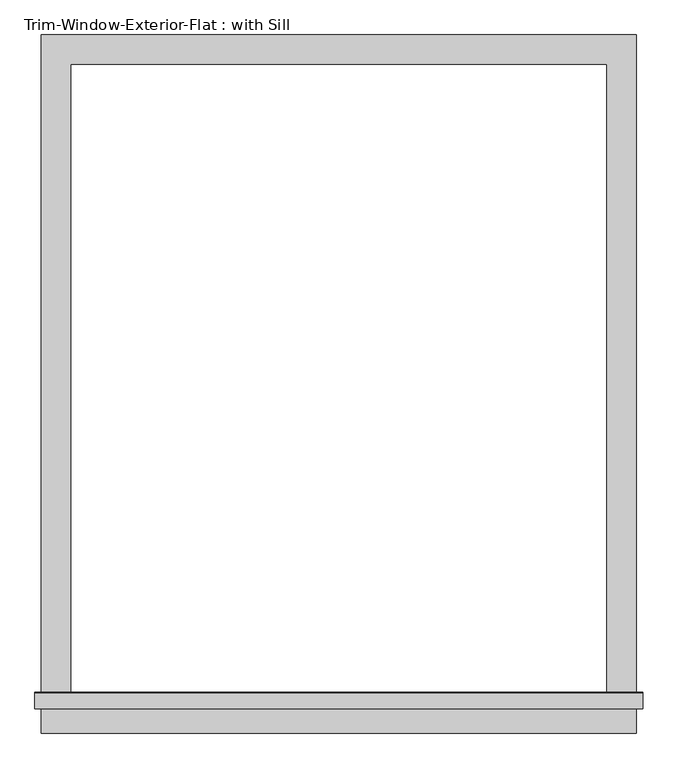
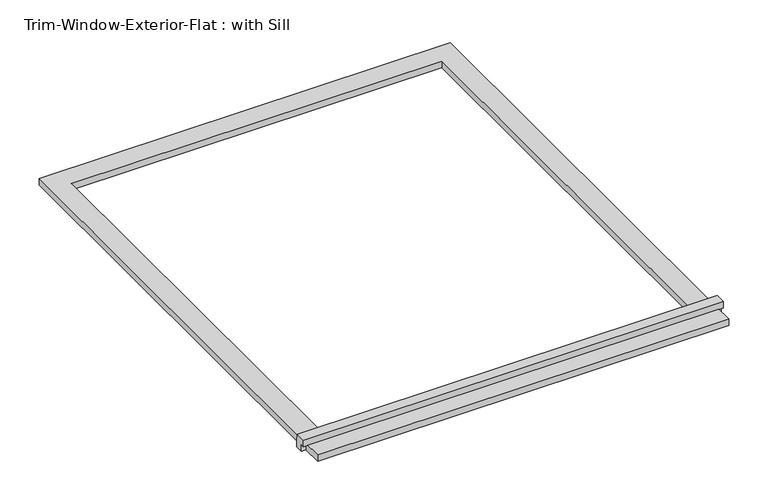
"""IFC4 building model written with IfcOpenShell, lengths in millimetres: proxy geometry, Trim-Window-Exterior-Flat : with Sill."""

from ifc_helpers import new_model, si_unit, frame, origin, origin_with_axes, place, context, project, spatial, polyline, outline, extrude, source, transform, mapped, element, save


def trim_window_exterior_flat_with_sill_29d7a895(model_context):
    return source(origin(), model_context, "Body", "SweptSolid", [
        extrude(outline(polyline([(577.85, -1241.3823709), (577.85, -1298.5323709), (-577.85, -1298.5323709), (-577.85, -1241.3823709), (577.85, -1241.3823709)])), origin_with_axes(), (0.0, 0.0, 1.0), 19.05),
        extrude(outline(polyline([(-1250.95, 38.1), (-1221.6580645, 38.1), (-1219.2, 19.05), (-1219.2, 0.0), (-1241.3823709, 0.0), (-1241.3823709, 19.05), (-1250.95, 19.05), (-1250.95, 38.1)])), frame((-590.55, 0.0, 0.0), z_axis=(1.0, 0.0, 0.0), x_axis=(0.0, 1.0, 0.0)), (0.0, 0.0, 1.0), 1181.1),
        extrude(outline(polyline([(-577.85, 57.15), (577.85, 57.15), (577.85, -1219.2), (520.7, -1219.2), (520.7, 0.0), (-520.7, 0.0), (-520.7, -1219.2), (-577.85, -1219.2), (-577.85, 57.15)])), origin_with_axes(), (0.0, 0.0, 1.0), 19.05),
    ])


if __name__ == "__main__":
    model = new_model("IFC4")
    model_context = context("Model", 3, world=origin())
    ifc_project = project(units=[si_unit("LENGTHUNIT", "METRE", prefix="MILLI")], contexts=[model_context])
    site = spatial("IfcSite", under=ifc_project)
    building = spatial("IfcBuilding", under=site)
    placement = place(None, origin())
    trim_window_exterior_flat_with_sill_shape = trim_window_exterior_flat_with_sill_29d7a895(model_context)
    element("IfcBuildingElementProxy", 1, Name="Trim-Window-Exterior-Flat : with Sill", ObjectType="Trim-Window-Exterior-Flat : with Sill", at=placement, inside=building, context=model_context, shape_type="MappedRepresentation", body=[
        mapped(trim_window_exterior_flat_with_sill_shape, transform((0.0, 0.0, 0.0), x_axis=(1.0, 0.0, 0.0), y_axis=(0.0, 1.0, 0.0), z_axis=(0.0, 0.0, 1.0))),
    ])
    save(model, "model.ifc")

# Revit data of these elements
# Type "Trim-Window-Exterior-Flat : with Sill"
#   Trim Width = 0' - 2 1/4"
#   Trim Thickness_Picture Frame = 0' - 1 1/4"
#   Trim Thickness_with Sill = 0' - 0 3/4"
#   Sill Thickness = 0' - 1 1/4"
#   Opening Width [instance default] = 2' - 0"
#   Opening Height [instance default] = 3' - 0"
#   Default Elevation = 4' - 0"
#   Sill = yes
#   Picture Frame = no
#   Trim Material [instance default] = none
# Element 1 (IfcBuildingElementProxy, "Trim-Window-Exterior-Flat : with Sill")
#   Opening Width = 3' - 5"
#   Opening Height = 4' - 0"
#   Trim Material = Clad - White
#   Materials on its faces: "Clad - White"
# Materials
#   "Clad - White": class "Wood", colour RGB 242 242 238, transparency 0, Cost = 0
